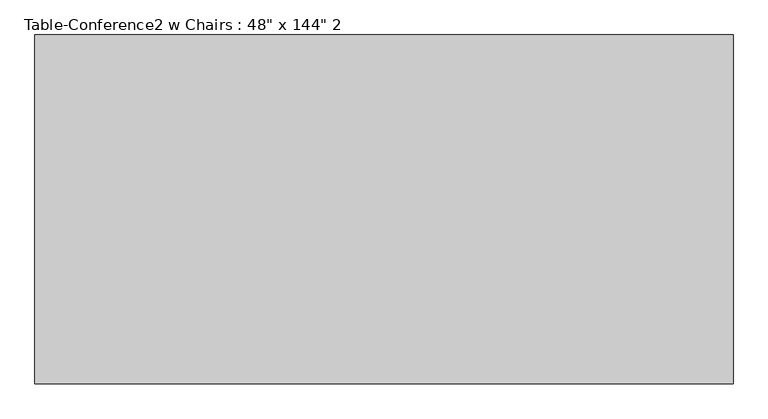
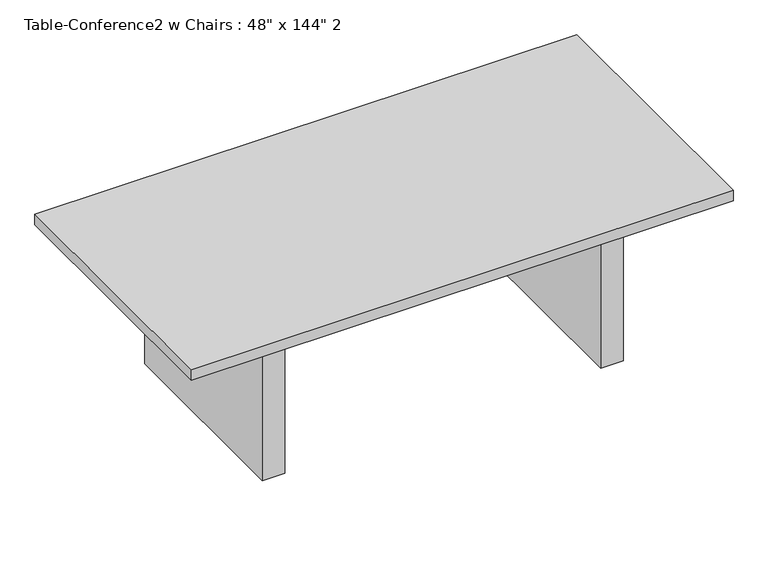
"""IFC4 building model written with IfcOpenShell, lengths in millimetres: furniture geometry."""

from ifc_helpers import new_model, si_unit, frame, origin, origin_with_axes, place, context, project, spatial, polyline, outline, extrude, source, transform, mapped, element, save


def furniture_6f689152(model_context):
    return source(origin(), model_context, "Body", "SweptSolid", [
        extrude(outline(polyline([(1219.2, -609.6), (-1219.2, -609.6), (-1219.2, 609.6), (1219.2, 609.6), (1219.2, -609.6)])), frame((0.0, 0.0, 711.2), z_axis=(0.0, 0.0, 1.0), x_axis=(1.0, 0.0, 0.0)), (0.0, 0.0, 1.0), 50.8),
        extrude(outline(polyline([(-711.2, -457.2), (-812.8, -457.2), (-812.8, 457.2), (-711.2, 457.2), (-711.2, -457.2)])), origin_with_axes(), (0.0, 0.0, 1.0), 711.2),
        extrude(outline(polyline([(812.8, -457.2), (711.2, -457.2), (711.2, 457.2), (812.8, 457.2), (812.8, -457.2)])), origin_with_axes(), (0.0, 0.0, 1.0), 711.2),
        extrude(outline(polyline([(711.2, 457.2), (711.2, 419.1), (-711.2, 419.1), (-711.2, 457.2), (711.2, 457.2)])), frame((0.0, 0.0, 609.6), z_axis=(0.0, 0.0, 1.0), x_axis=(1.0, 0.0, 0.0)), (0.0, 0.0, 1.0), 101.6),
        extrude(outline(polyline([(711.2, -457.2), (-711.2, -457.2), (-711.2, -419.1), (711.2, -419.1), (711.2, -457.2)])), frame((0.0, 0.0, 609.6), z_axis=(0.0, 0.0, 1.0), x_axis=(1.0, 0.0, 0.0)), (0.0, 0.0, 1.0), 101.6),
    ])


if __name__ == "__main__":
    model = new_model("IFC4")
    model_context = context("Model", 3, world=origin())
    ifc_project = project(units=[si_unit("LENGTHUNIT", "METRE", prefix="MILLI")], contexts=[model_context])
    site = spatial("IfcSite", under=ifc_project)
    building = spatial("IfcBuilding", under=site)
    placement = place(None, origin())
    furniture_shape = furniture_6f689152(model_context)
    element("IfcFurniture", 1, ObjectType="Table-Conference2 w Chairs : 48\" x 144\" 2", at=placement, inside=building, context=model_context, shape_type="MappedRepresentation", body=[
        mapped(furniture_shape, transform((0.0, 0.0, 0.0), x_axis=(1.0, 0.0, 0.0), y_axis=(0.0, 1.0, 0.0), z_axis=(0.0, 0.0, 1.0))),
    ])
    save(model, "model.ifc")

# Revit data of these elements
# Type "Table-Conference2 w Chairs : 48\" x 144\" 2"
#   Assembly Code = "E2020200"
#   Description = "Seating 12-14"
#   Height = 2' - 6"
#   Length = 8' - 0"
#   Width = 4' - 0"
#   Number Of Chairs One Side = 3
#   Number Of Chairs = 8
#   Material = Wood - Cherry
#   Default Elevation = 0
# Element 1 (IfcFurniture, "Table-Conference2 w Chairs : 48\" x 144\" 2")
#   Materials on its faces: "Wood - Cherry"
# Materials
#   "Wood - Cherry": colour RGB 151 75 0, transparency 0
